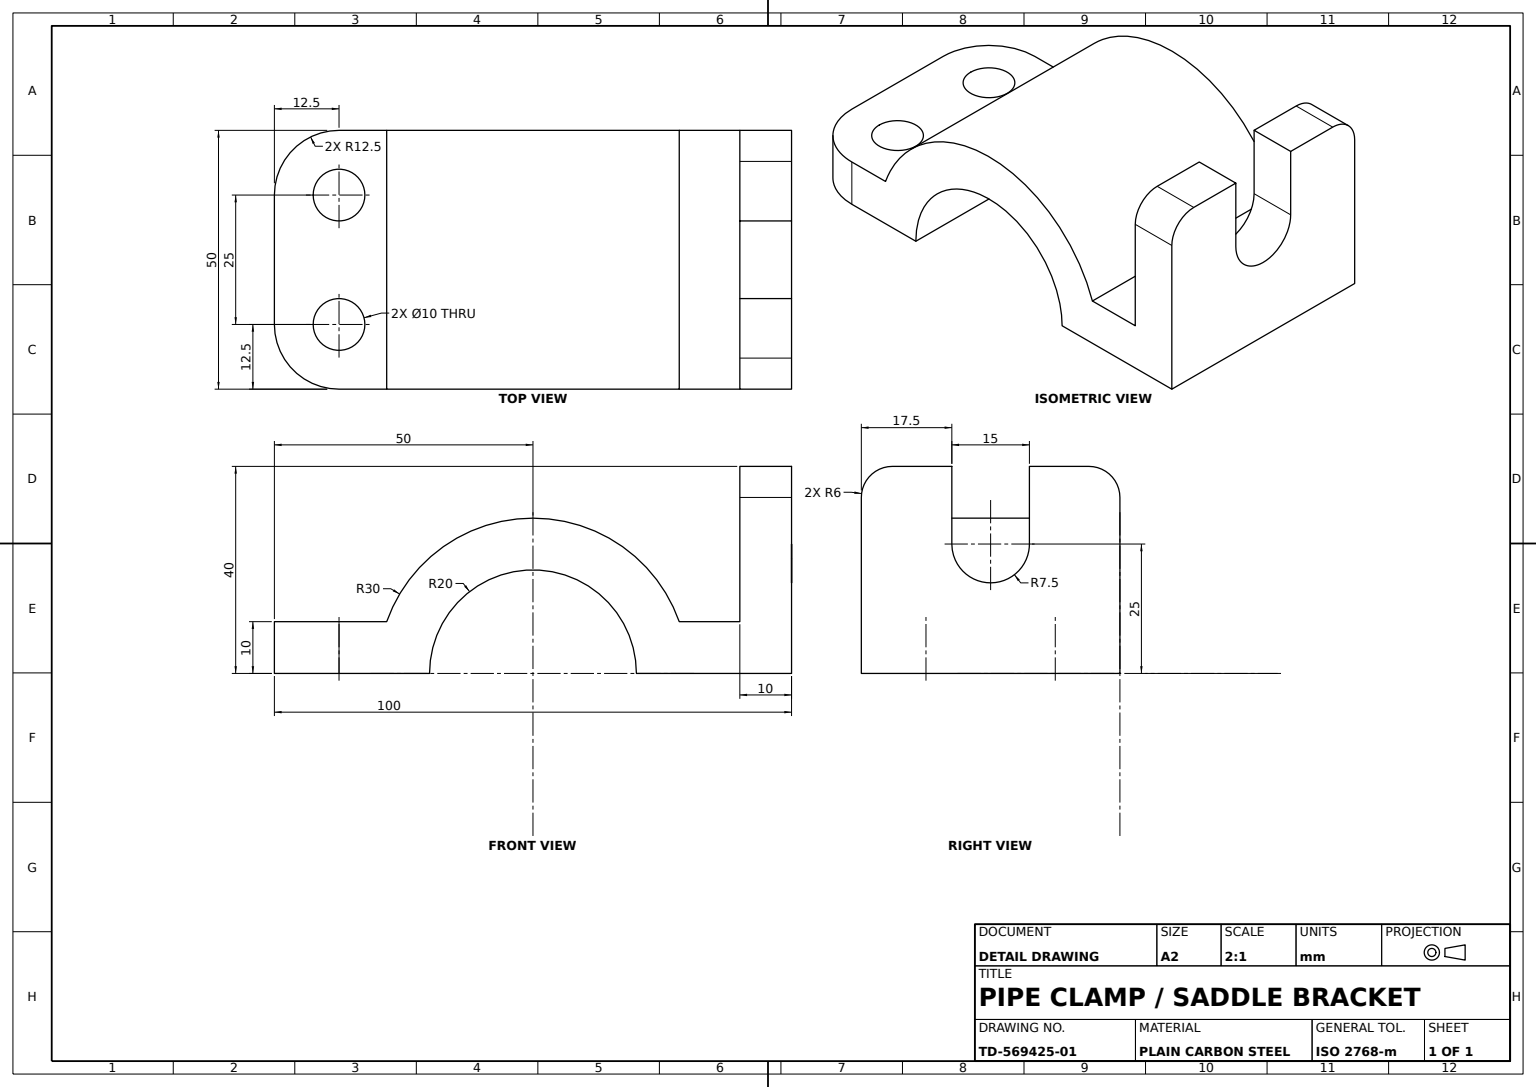
SolidWorks part; units mm, degrees
material "Plain Carbon Steel"
ref_plane "Front Plane" through (0, 0, 0) normal (0, 0, 1) x (1, 0, 0)
ref_plane "Top Plane" through (0, 0, 0) normal (0, 1, 0) x (1, 0, 0)
ref_plane "Right Plane" through (0, 0, 0) normal (1, 0, 0) x (0, 0, -1)
sketch "Base Profile Sketch" plane through (0, 0, 0) normal (0, 0, 1) x (1, 0, 0)
  line L1 (50, 40) -> (50, 0)
  line L2 (50, 0) -> (20, 0)
  line L3 (-20, 0) -> (-50, 0)
  line L4 (-50, 0) -> (-50, 10)
  line L5 (-50, 10) -> (-28.2843, 10)
  line L6 (0, 0) -> (0, 61.5791) construction
  line L7 (50, 40) -> (40, 40)
  line L8 (40, 40) -> (40, 10)
  line L9 (40, 10) -> (28.2843, 10)
  arc A2 (-20, 0) -> (20, 0) centre (0, 0) cw
  arc A3 (-28.2843, 10) -> (28.2843, 10) centre (0, 0) cw
  dimension "D1" = 40
  dimension "D3" = 30
  dimension "D5" = 10
  dimension "D6" = 20
  dimension "D7" = 10
  dimension "D2" = 10
  dimension "D4" = 100
  dimension "D8" = 40
extrude "Base Body Extrude" add sketch "Base Profile Sketch" along normal mid plane 50
fillet "Flange End Rounds R12.5" radius 12.5 2 edges at (-50, 5, -25) (-50, 5, 25)
fillet "Edge Fillets R6" radius 6 2 edges at (45, 40, -25) (45, 40, 25)
sketch "Flange Holes Sketch" plane through (0, 10, 0) normal (0, 1, 0) x (1, 0, 0)
  circle A0 centre (-37.5, -12.5) radius 5
  circle A1 centre (-37.5, 12.5) radius 5
  dimension "D1" = 10
extrude "Flange Bolt Holes 2x" cut sketch "Flange Holes Sketch" against normal through all both and the other way through all
sketch "Fork Slot Sketch" plane through (50, 0, 0) normal (1, 0, 0) x (0, 0, -1)
  line L0 (0, 0) -> (0, 40) construction
  line L1 (-19, 40) -> (19, 40) construction
  line L2 (7.5, 40) -> (7.5, 25)
  line L3 (-7.5, 40) -> (-7.5, 25)
  line L4 (-25, 0) -> (25, 0) construction
  line L5 (-7.5, 40) -> (7.5, 40)
  arc A0 (-7.5, 25) -> (7.5, 25) centre (0, 25) ccw
  dimension "D1" = 15
  dimension "D2" = 25
extrude "Fork Slot" cut sketch "Fork Slot Sketch" against normal up to next and the other way through all
